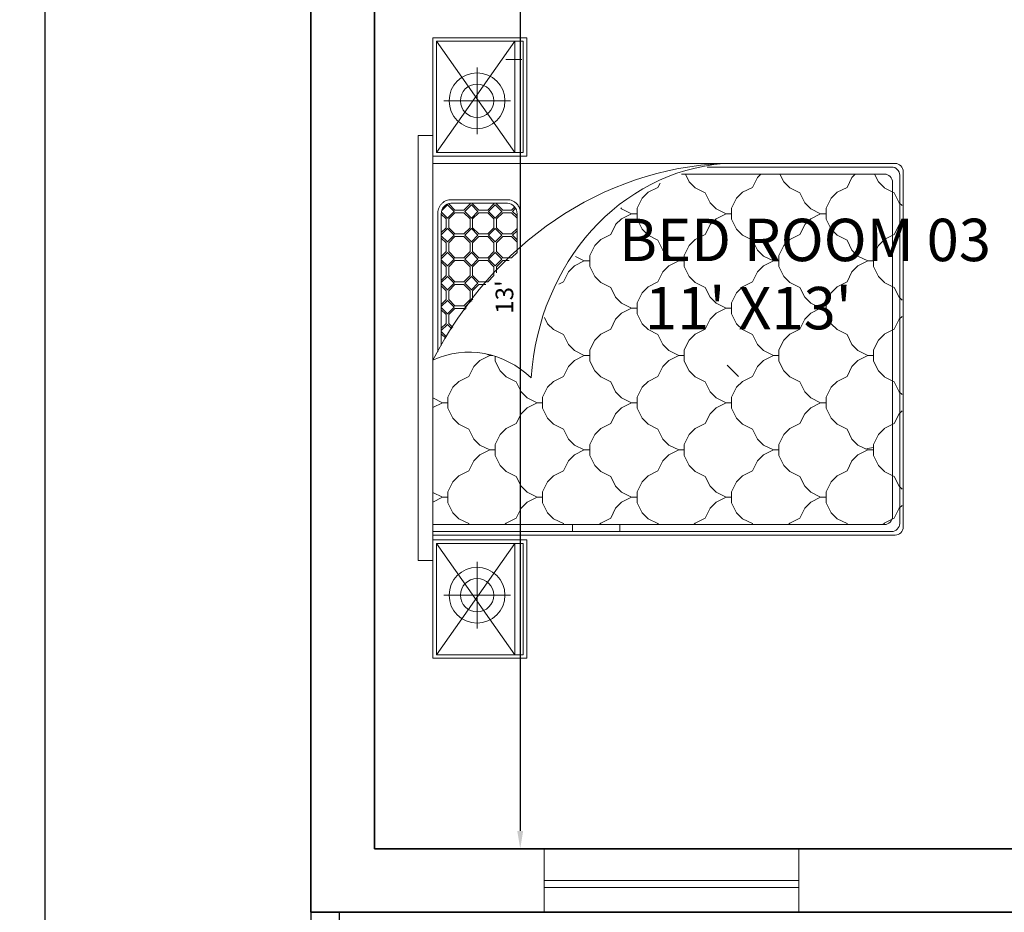
# Model space of a CAD drawing. Units: inches. Extents: x 2025 to 2528, y 1525 to 2336.
# Tile 2 of 18: x 2025 to 2164, y 1704 to 1831. Entities that reach past the tile are written whole.
import ezdxf

# ---------------------------------------------------------------- set-up
doc = ezdxf.new("R2010")
doc.units = ezdxf.units.IN
for name, color, linetype, lineweight in [('A-ANNO-DIMS', 2, 'Continuous', 18), ('A-AREA-IDEN', 7, 'Continuous', 25), ('A-FLOR', 7, 'Continuous', 25), ('A-FURN', 8, 'Continuous', 18), ('A-GLAZ', 4, 'Continuous', 18), ('A-WALL', 7, 'Continuous', 35)]:
    doc.layers.add(name, color=color, linetype=linetype, lineweight=lineweight)
doc.styles.get("Standard").update_dxf_attribs({"font": 'arial.ttf'})
doc.dimstyles.new('Copy of ISO-25', dxfattribs={"dimtxt": 2.5, "dimasz": 2.5, "dimexe": 1.25, "dimexo": 0.625, "dimtad": 1, "dimdec": 1, "dimlunit": 4, "dimtxsty": 'Standard', "dimcen": 2.5, "dimadec": 0, "dimazin": 0, "dimtfac": 1, "dimtdec": 1, "dimtmove": 0, "dimatfit": 3, "dimfxl": 1, "dimarcsym": 0})

# ---------------------------------------------------------------- blocks, each defined once
blk = doc.blocks.new('*D30')
at = {"layer": 'A-ANNO-DIMS', "color": 0, "lineweight": -2, "transparency": 16777216}
for p, q in [((2078.14, 1869.41), (2096.86, 1869.41)), ((2095.61, 1866.91), (2095.61, 1715.91)), ((2075.64, 1713.41), (2096.86, 1713.41))]:
    blk.add_line(p, q, dxfattribs=at)
at = {"layer": 'A-ANNO-DIMS', "color": 0, "transparency": 16777216}
for points in [[(2095.2, 1866.91), (2096.03, 1866.91), (2095.61, 1869.41)], [(2095.2, 1715.91), (2096.03, 1715.91), (2095.61, 1713.41)]]:
    blk.add_solid(points, dxfattribs=at)
at = {"layer": 'Defpoints', "color": 0, "transparency": 16777216}
for p in [(2077.51, 1869.41), (2075.01, 1713.41), (2095.61, 1713.41)]:
    blk.add_point(p, dxfattribs=at)
at = {"layer": 'A-ANNO-DIMS', "color": 0, "transparency": 16777216, "insert": (2093.71, 1791.41), "char_height": 2.5, "attachment_point": 5, "rotation": 90}
blk.add_mtext("13'", dxfattribs=at)
blk = doc.blocks.new('A$C029D5C69')
for p, q in [((0.4164, 2.0693), (0.4164, 2.0066)), ((2.2315, 2.0693), (0.4164, 2.0693)), ((2.2315, 2.0066), (2.2315, 2.0693)), ((0, 1.606), (0, 2.0066)), ((0, 2.0066), (0.505, 2.0066)), ((0.0151, 1.6211), (0.0151, 1.9915)), ((0.0151, 1.9915), (0.4899, 1.9915)), ((0.4164, 2.0066), (2.2315, 2.0066)), ((0.4899, 1.9915), (0.4899, 1.6211)), ((0.505, 2.0066), (0.505, 1.606)), ((0.5252, 0.0351), (0.5252, 2.0066)), ((0.5403, 0.0502), (0.5403, 2.0066)), ((0.5706, 0.0805), (0.5706, 2.0066)), ((0.6869, 1.966), (0.6666, 2.0066)), ((0.7072, 2.0066), (0.6869, 1.966)), ((1.0902, 1.966), (1.0699, 2.0066)), ((1.1106, 2.0066), (1.0902, 1.966)), ((1.8954, 1.9865), (1.3081, 1.9865)), ((2.1114, 2.0087), (2.1114, 0.0351)), ((2.6479, 2.0066), (2.1429, 2.0066)), ((2.1429, 2.0066), (2.1429, 1.606)), ((2.6328, 1.9915), (2.158, 1.9915)), ((2.158, 1.9915), (2.158, 1.6211)), ((2.6328, 1.6211), (2.6328, 1.9915)), ((2.6479, 1.606), (2.6479, 2.0066)), ((0.2689, 1.9609), (0.2689, 1.6764)), ((0.6634, 1.9425), (0.621, 1.9213)), ((0.6634, 1.9425), (0.621, 1.9213)), ((0.6869, 1.9425), (0.6634, 1.9425)), ((0.6869, 1.9425), (0.6869, 1.966)), ((0.6869, 1.9425), (0.6869, 1.966)), ((0.6869, 1.9425), (0.7104, 1.9425)), ((0.7528, 1.9213), (0.7104, 1.9425)), ((0.7528, 1.9213), (0.7104, 1.9425)), ((1.0668, 1.9425), (1.0244, 1.9213)), ((1.0668, 1.9425), (1.0244, 1.9213)), ((1.0902, 1.9425), (1.0668, 1.9425)), ((1.0902, 1.9425), (1.0902, 1.966)), ((1.0902, 1.9425), (1.0902, 1.966)), ((1.0902, 1.9425), (1.1137, 1.9425)), ((1.1561, 1.9213), (1.1137, 1.9425)), ((1.1561, 1.9213), (1.1137, 1.9425)), ((1.8954, 1.9713), (1.3339, 1.9713)), ((1.3849, 1.9713), (1.3656, 1.952)), ((1.3945, 1.9713), (1.3714, 1.9483)), ((1.4249, 1.945), (1.3986, 1.9713)), ((1.4249, 1.945), (1.4059, 1.926)), ((1.4288, 1.9507), (1.4081, 1.9713)), ((1.4288, 1.9394), (1.4116, 1.9222)), ((1.4476, 1.9507), (1.4288, 1.9507)), ((1.4288, 1.9393), (1.4476, 1.9393)), ((1.4476, 1.9507), (1.4664, 1.9507)), ((1.4664, 1.9393), (1.4476, 1.9393)), ((1.487, 1.9713), (1.4664, 1.9507)), ((1.493, 1.9128), (1.4664, 1.9394)), ((1.4966, 1.9713), (1.4703, 1.945)), ((1.4986, 1.9167), (1.4703, 1.945)), ((1.527, 1.945), (1.4986, 1.9167)), ((1.527, 1.945), (1.5007, 1.9713)), ((1.5309, 1.9394), (1.5043, 1.9128)), ((1.5309, 1.9507), (1.5102, 1.9713)), ((1.5497, 1.9507), (1.5309, 1.9507)), ((1.5309, 1.9393), (1.5497, 1.9393)), ((1.5497, 1.9507), (1.5685, 1.9507)), ((1.5685, 1.9393), (1.5497, 1.9393)), ((1.5891, 1.9713), (1.5685, 1.9507)), ((1.595, 1.9128), (1.5685, 1.9394)), ((1.5987, 1.9713), (1.5724, 1.945)), ((1.6007, 1.9167), (1.5724, 1.945)), ((1.6291, 1.945), (1.6007, 1.9167)), ((1.6291, 1.945), (1.6028, 1.9713)), ((1.633, 1.9394), (1.6064, 1.9128)), ((1.633, 1.9507), (1.6123, 1.9713)), ((1.6518, 1.9507), (1.633, 1.9507)), ((1.633, 1.9393), (1.6518, 1.9393)), ((1.6518, 1.9507), (1.6706, 1.9507)), ((1.6706, 1.9393), (1.6518, 1.9393)), ((1.6912, 1.9713), (1.6706, 1.9507)), ((1.6971, 1.9128), (1.6706, 1.9394)), ((1.7008, 1.9713), (1.6745, 1.945)), ((1.7028, 1.9167), (1.6745, 1.945)), ((1.7312, 1.945), (1.7028, 1.9167)), ((1.7312, 1.945), (1.7049, 1.9713)), ((1.7351, 1.9394), (1.7085, 1.9128)), ((1.7351, 1.9507), (1.7144, 1.9713)), ((1.7539, 1.9507), (1.7351, 1.9507)), ((1.7351, 1.9393), (1.7539, 1.9393)), ((1.7539, 1.9507), (1.7727, 1.9507)), ((1.7727, 1.9393), (1.7539, 1.9393)), ((1.7933, 1.9713), (1.7727, 1.9507)), ((1.7992, 1.9128), (1.7727, 1.9394)), ((1.8029, 1.9713), (1.7766, 1.945)), ((1.8049, 1.9167), (1.7766, 1.945)), ((1.8333, 1.945), (1.8049, 1.9167)), ((1.8333, 1.945), (1.807, 1.9713)), ((1.8372, 1.9394), (1.8106, 1.9128)), ((1.8372, 1.9507), (1.8165, 1.9713)), ((1.856, 1.9507), (1.8372, 1.9507)), ((1.8372, 1.9393), (1.856, 1.9393)), ((1.856, 1.9507), (1.8748, 1.9507)), ((1.8748, 1.9393), (1.856, 1.9393)), ((1.8954, 1.9713), (1.8748, 1.9507)), ((1.9013, 1.9128), (1.8748, 1.9394)), ((1.9043, 1.9707), (1.8787, 1.945)), ((1.907, 1.9167), (1.8787, 1.945)), ((1.9354, 1.945), (1.907, 1.9167)), ((1.9354, 1.945), (1.9114, 1.969)), ((1.9393, 1.9394), (1.9127, 1.9128)), ((1.9393, 1.9393), (1.9404, 1.9393)), ((2.379, 1.9609), (2.379, 1.6764)), ((0.5955, 1.8958), (0.5743, 1.8534)), ((0.621, 1.9213), (0.5955, 1.8958)), ((0.7783, 1.8958), (0.7528, 1.9213)), ((0.7995, 1.8534), (0.7783, 1.8958)), ((0.9989, 1.8958), (0.9777, 1.8534)), ((1.0243, 1.9213), (0.9988, 1.8958)), ((1.1816, 1.8958), (1.1561, 1.9213)), ((1.2028, 1.8534), (1.1816, 1.8958)), ((1.493, 1.8752), (1.493, 1.9128)), ((1.5043, 1.8752), (1.5043, 1.9128)), ((1.595, 1.8752), (1.595, 1.9128)), ((1.6064, 1.8752), (1.6064, 1.9128)), ((1.6971, 1.8752), (1.6971, 1.9128)), ((1.7085, 1.8752), (1.7085, 1.9128)), ((1.7992, 1.8752), (1.7992, 1.9128)), ((1.8106, 1.8752), (1.8106, 1.9128)), ((1.9013, 1.8752), (1.9013, 1.9128)), ((1.9127, 1.8752), (1.9127, 1.9128)), ((1.9414, 1.688), (1.9414, 1.931)), ((1.9565, 1.688), (1.9565, 1.931)), ((0.5743, 1.8534), (0.5706, 1.8515)), ((0.5743, 1.8534), (0.5706, 1.8515)), ((0.8419, 1.8322), (0.7995, 1.8534)), ((0.8419, 1.8322), (0.7995, 1.8534)), ((0.9777, 1.8534), (0.9353, 1.8322)), ((0.9777, 1.8534), (0.9353, 1.8322)), ((1.2452, 1.8322), (1.2028, 1.8534)), ((1.2452, 1.8322), (1.2028, 1.8534)), ((1.493, 1.8752), (1.4867, 1.869)), ((1.4986, 1.8713), (1.4922, 1.8648)), ((1.527, 1.8429), (1.4986, 1.8713)), ((1.5309, 1.8486), (1.5043, 1.8752)), ((1.5497, 1.8486), (1.5309, 1.8486)), ((1.5497, 1.8486), (1.5685, 1.8486)), ((1.595, 1.8752), (1.5685, 1.8486)), ((1.6007, 1.8713), (1.5724, 1.8429)), ((1.6291, 1.8429), (1.6007, 1.8713)), ((1.633, 1.8486), (1.6064, 1.8752)), ((1.6518, 1.8486), (1.633, 1.8486)), ((1.6518, 1.8486), (1.6706, 1.8486)), ((1.6971, 1.8752), (1.6706, 1.8486)), ((1.7028, 1.8713), (1.6745, 1.8429)), ((1.7312, 1.8429), (1.7028, 1.8713)), ((1.7351, 1.8486), (1.7085, 1.8752)), ((1.7539, 1.8486), (1.7351, 1.8486)), ((1.7539, 1.8486), (1.7727, 1.8486)), ((1.7992, 1.8752), (1.7727, 1.8486)), ((1.8049, 1.8713), (1.7766, 1.8429)), ((1.8333, 1.8429), (1.8049, 1.8713)), ((1.8372, 1.8486), (1.8106, 1.8752)), ((1.856, 1.8486), (1.8372, 1.8486)), ((1.856, 1.8486), (1.8748, 1.8486)), ((1.9013, 1.8752), (1.8748, 1.8486)), ((1.907, 1.8713), (1.8787, 1.8429)), ((1.9354, 1.8429), (1.907, 1.8713)), ((1.9393, 1.8486), (1.9127, 1.8752)), ((1.9414, 1.8486), (1.9393, 1.8486)), ((0.1267, 1.8186), (0.4111, 1.8186)), ((0.8674, 1.8067), (0.8419, 1.8322)), ((0.8886, 1.7643), (0.8674, 1.8067)), ((0.9098, 1.8067), (0.8886, 1.7643)), ((0.9352, 1.8322), (0.9097, 1.8067)), ((1.2707, 1.8067), (1.2452, 1.8322)), ((1.2919, 1.7643), (1.2707, 1.8067)), ((1.527, 1.8429), (1.5242, 1.8401)), ((1.5309, 1.8373), (1.5295, 1.8359)), ((1.5309, 1.8373), (1.5497, 1.8373)), ((1.5685, 1.8373), (1.5497, 1.8373)), ((1.595, 1.8107), (1.5685, 1.8373)), ((1.6007, 1.8146), (1.5724, 1.8429)), ((1.595, 1.7806), (1.595, 1.8107)), ((1.6291, 1.8429), (1.6007, 1.8146)), ((1.633, 1.8373), (1.6064, 1.8107)), ((1.6064, 1.7731), (1.6064, 1.8107)), ((1.633, 1.8373), (1.6518, 1.8373)), ((1.6706, 1.8373), (1.6518, 1.8373)), ((1.6971, 1.8107), (1.6706, 1.8373)), ((1.7028, 1.8146), (1.6745, 1.8429)), ((1.6971, 1.7731), (1.6971, 1.8107)), ((1.7312, 1.8429), (1.7028, 1.8146)), ((1.7351, 1.8373), (1.7085, 1.8107)), ((1.7085, 1.7731), (1.7085, 1.8107)), ((1.7351, 1.8373), (1.7539, 1.8373)), ((1.7727, 1.8373), (1.7539, 1.8373)), ((1.7992, 1.8107), (1.7727, 1.8373)), ((1.8049, 1.8146), (1.7766, 1.8429)), ((1.7992, 1.7731), (1.7992, 1.8107)), ((1.8333, 1.8429), (1.8049, 1.8146)), ((1.8372, 1.8373), (1.8106, 1.8107)), ((1.8106, 1.7731), (1.8106, 1.8107)), ((1.8372, 1.8373), (1.856, 1.8373)), ((1.8748, 1.8373), (1.856, 1.8373)), ((1.9013, 1.8107), (1.8748, 1.8373)), ((1.907, 1.8146), (1.8787, 1.8429)), ((1.9013, 1.7731), (1.9013, 1.8107)), ((1.9354, 1.8429), (1.907, 1.8146)), ((1.9393, 1.8373), (1.9127, 1.8107)), ((1.9127, 1.7731), (1.9127, 1.8107)), ((1.9393, 1.8373), (1.9414, 1.8373)), ((2.2367, 1.8186), (2.5212, 1.8186)), ((1.2981, 1.7768), (1.2919, 1.7643)), ((1.633, 1.7465), (1.6064, 1.7731)), ((1.6971, 1.7731), (1.6706, 1.7465)), ((1.7028, 1.7692), (1.6745, 1.7408)), ((1.7312, 1.7408), (1.7028, 1.7692)), ((1.7351, 1.7465), (1.7085, 1.7731)), ((1.7992, 1.7731), (1.7727, 1.7465)), ((1.8049, 1.7692), (1.7766, 1.7408)), ((1.8333, 1.7408), (1.8049, 1.7692)), ((1.8372, 1.7465), (1.8106, 1.7731)), ((1.9013, 1.7731), (1.8748, 1.7465)), ((1.907, 1.7692), (1.8787, 1.7408)), ((1.9354, 1.7408), (1.907, 1.7692)), ((1.9393, 1.7465), (1.9127, 1.7731)), ((0.8651, 1.7408), (0.8227, 1.7196)), ((0.8651, 1.7408), (0.8227, 1.7196)), ((0.912, 1.7408), (0.8651, 1.7408)), ((0.8886, 1.7408), (0.8886, 1.7643)), ((0.9544, 1.7196), (0.912, 1.7408)), ((0.9544, 1.7196), (0.912, 1.7408)), ((1.2684, 1.7408), (1.226, 1.7196)), ((1.2684, 1.7408), (1.226, 1.7196)), ((1.2885, 1.7408), (1.2684, 1.7408)), ((1.2919, 1.7519), (1.2919, 1.7643)), ((1.6518, 1.7465), (1.633, 1.7465)), ((1.6443, 1.7352), (1.6518, 1.7352)), ((1.6518, 1.7465), (1.6706, 1.7465)), ((1.6706, 1.7352), (1.6518, 1.7352)), ((1.6971, 1.7086), (1.6706, 1.7352)), ((1.7028, 1.7125), (1.6745, 1.7408)), ((1.7312, 1.7408), (1.7028, 1.7125)), ((1.7351, 1.7352), (1.7085, 1.7086)), ((1.7539, 1.7465), (1.7351, 1.7465)), ((1.7351, 1.7352), (1.7539, 1.7352)), ((1.7539, 1.7465), (1.7727, 1.7465)), ((1.7727, 1.7352), (1.7539, 1.7352)), ((1.7992, 1.7086), (1.7727, 1.7352)), ((1.8049, 1.7125), (1.7766, 1.7408)), ((1.8333, 1.7408), (1.8049, 1.7125)), ((1.8372, 1.7352), (1.8106, 1.7086)), ((1.856, 1.7465), (1.8372, 1.7465)), ((1.8372, 1.7352), (1.856, 1.7352)), ((1.856, 1.7465), (1.8748, 1.7465)), ((1.8748, 1.7352), (1.856, 1.7352)), ((1.9013, 1.7086), (1.8748, 1.7352)), ((1.907, 1.7125), (1.8787, 1.7408)), ((1.9354, 1.7408), (1.907, 1.7125)), ((1.9393, 1.7352), (1.9127, 1.7086)), ((1.9414, 1.7465), (1.9393, 1.7465)), ((1.9393, 1.7352), (1.9414, 1.7352)), ((0.5766, 1.6941), (0.5706, 1.7002)), ((0.5978, 1.6517), (0.5766, 1.6941)), ((0.7972, 1.6941), (0.776, 1.6517)), ((0.8227, 1.7196), (0.7972, 1.6941)), ((0.98, 1.6941), (0.9545, 1.7196)), ((1.0011, 1.6517), (0.9799, 1.6941)), ((1.2005, 1.6941), (1.1793, 1.6517)), ((1.226, 1.7196), (1.2005, 1.6941)), ((1.6971, 1.682), (1.6971, 1.7086)), ((1.7085, 1.671), (1.7085, 1.7086)), ((1.7992, 1.671), (1.7992, 1.7086)), ((1.8106, 1.671), (1.8106, 1.7086)), ((1.9013, 1.671), (1.9013, 1.7086)), ((1.9127, 1.671), (1.9127, 1.7086)), ((2.5551, 1.6275), (2.5551, 1.696)), ((0.6402, 1.6305), (0.5978, 1.6517)), ((0.6402, 1.6305), (0.5978, 1.6517)), ((0.776, 1.6517), (0.7336, 1.6305)), ((0.776, 1.6517), (0.7336, 1.6305)), ((1.0435, 1.6305), (1.0011, 1.6517)), ((1.0435, 1.6305), (1.0011, 1.6517)), ((1.1793, 1.6517), (1.1369, 1.6305)), ((1.1793, 1.6517), (1.1369, 1.6305)), ((1.7318, 1.6477), (1.7085, 1.671)), ((1.8961, 1.6477), (1.7289, 1.6477)), ((1.7992, 1.671), (1.7759, 1.6477)), ((1.8049, 1.6671), (1.7855, 1.6477)), ((1.8244, 1.6477), (1.8049, 1.6671)), ((1.8339, 1.6477), (1.8106, 1.671)), ((1.9013, 1.671), (1.878, 1.6477)), ((1.907, 1.6671), (1.8876, 1.6477)), ((1.9202, 1.6539), (1.907, 1.6671)), ((1.926, 1.6577), (1.9127, 1.671)), ((0.505, 1.606), (0, 1.606)), ((0.4899, 1.6211), (0.0151, 1.6211)), ((0.6657, 1.605), (0.6402, 1.6305)), ((0.6869, 1.5626), (0.6657, 1.605)), ((0.7081, 1.605), (0.6869, 1.5626)), ((0.7336, 1.6305), (0.7081, 1.605)), ((1.0691, 1.605), (1.0436, 1.6305)), ((1.0902, 1.5626), (1.069, 1.605)), ((1.1114, 1.605), (1.0902, 1.5626)), ((1.1369, 1.6305), (1.1114, 1.605)), ((1.8961, 1.6325), (1.7422, 1.6325)), ((2.1429, 1.606), (2.6479, 1.606)), ((2.158, 1.6211), (2.6328, 1.6211)), ((0.6869, 1.5392), (0.6869, 1.5626)), ((0.6869, 1.5392), (0.6869, 1.5626)), ((1.0902, 1.5392), (1.0902, 1.5626)), ((1.0902, 1.5392), (1.0902, 1.5626)), ((0.621, 1.5179), (0.5955, 1.4924)), ((0.6634, 1.5391), (0.621, 1.5179)), ((0.6634, 1.5391), (0.621, 1.5179)), ((0.6869, 1.5392), (0.6634, 1.5392)), ((0.6869, 1.5392), (0.7104, 1.5392)), ((0.7528, 1.5179), (0.7104, 1.5391)), ((0.7528, 1.5179), (0.7104, 1.5391)), ((0.7783, 1.4924), (0.7528, 1.5179)), ((1.0243, 1.5179), (0.9988, 1.4924)), ((1.0668, 1.5391), (1.0244, 1.5179)), ((1.0668, 1.5391), (1.0244, 1.5179)), ((1.0902, 1.5392), (1.0668, 1.5392)), ((1.0902, 1.5392), (1.1137, 1.5392)), ((1.1561, 1.5179), (1.1137, 1.5391)), ((1.1561, 1.5179), (1.1137, 1.5391)), ((1.1816, 1.4924), (1.1561, 1.5179)), ((1.4277, 1.5179), (1.4022, 1.4924)), ((1.4534, 1.5308), (1.4277, 1.5179)), ((1.4534, 1.5308), (1.4277, 1.5179)), ((0.5955, 1.4925), (0.5743, 1.4501)), ((0.7995, 1.4501), (0.7783, 1.4925)), ((0.9989, 1.4925), (0.9777, 1.4501)), ((1.2028, 1.4501), (1.1816, 1.4925)), ((1.4022, 1.4925), (1.381, 1.4501)), ((0.5743, 1.45), (0.5706, 1.4481)), ((0.5743, 1.45), (0.5706, 1.4481)), ((0.8419, 1.4288), (0.7995, 1.45)), ((0.8419, 1.4288), (0.7995, 1.45)), ((0.8674, 1.4033), (0.8419, 1.4288)), ((0.9352, 1.4288), (0.9097, 1.4033)), ((0.9777, 1.45), (0.9353, 1.4288)), ((0.9777, 1.45), (0.9353, 1.4288)), ((1.2452, 1.4288), (1.2028, 1.45)), ((1.2452, 1.4288), (1.2028, 1.45)), ((1.2707, 1.4033), (1.2452, 1.4288)), ((1.3386, 1.4288), (1.3131, 1.4033)), ((1.381, 1.45), (1.3386, 1.4288)), ((1.381, 1.45), (1.3386, 1.4288)), ((1.6062, 1.4501), (1.5966, 1.4692)), ((1.6486, 1.4288), (1.6062, 1.45)), ((1.6486, 1.4288), (1.6062, 1.45)), ((1.6741, 1.4033), (1.6486, 1.4288)), ((0.5403, 1.4117), (0.5706, 1.4117)), ((0.8886, 1.361), (0.8674, 1.4034)), ((0.9098, 1.4034), (0.8886, 1.361)), ((1.2919, 1.361), (1.2707, 1.4034)), ((1.3131, 1.4034), (1.2919, 1.361)), ((1.6953, 1.361), (1.6741, 1.4034)), ((1.714, 1.3984), (1.6953, 1.361)), ((0.8886, 1.3375), (0.8886, 1.3609)), ((1.2919, 1.3375), (1.2919, 1.3609)), ((1.6953, 1.3375), (1.6953, 1.3609)), ((0.8227, 1.3163), (0.7972, 1.2908)), ((0.8651, 1.3374), (0.8227, 1.3162)), ((0.8651, 1.3374), (0.8227, 1.3162)), ((0.912, 1.3375), (0.8651, 1.3375)), ((0.9544, 1.3162), (0.912, 1.3374)), ((0.9544, 1.3162), (0.912, 1.3374)), ((0.98, 1.2908), (0.9545, 1.3163)), ((1.226, 1.3163), (1.2005, 1.2908)), ((1.2684, 1.3374), (1.226, 1.3162)), ((1.2684, 1.3374), (1.226, 1.3162)), ((1.3154, 1.3375), (1.2684, 1.3375)), ((1.3578, 1.3162), (1.3154, 1.3374)), ((1.3578, 1.3162), (1.3154, 1.3374)), ((1.3833, 1.2908), (1.3578, 1.3163)), ((1.6294, 1.3163), (1.6039, 1.2908)), ((1.6718, 1.3374), (1.6294, 1.3162)), ((1.6718, 1.3374), (1.6294, 1.3162)), ((1.7187, 1.3375), (1.6718, 1.3375)), ((1.7611, 1.3162), (1.7187, 1.3374)), ((1.7611, 1.3162), (1.7187, 1.3374)), ((1.7867, 1.2908), (1.7611, 1.3163)), ((0.5766, 1.2908), (0.5706, 1.2968)), ((0.5978, 1.2484), (0.5766, 1.2908)), ((0.7972, 1.2908), (0.776, 1.2484)), ((1.0011, 1.2484), (0.9799, 1.2908)), ((1.2005, 1.2908), (1.1793, 1.2484)), ((1.4045, 1.2484), (1.3833, 1.2908)), ((1.6039, 1.2908), (1.5827, 1.2484)), ((1.8078, 1.2484), (1.7866, 1.2908)), ((0.6402, 1.2271), (0.5978, 1.2483)), ((0.6402, 1.2271), (0.5978, 1.2483)), ((0.6657, 1.2017), (0.6402, 1.2272)), ((0.7336, 1.2272), (0.7081, 1.2017)), ((0.776, 1.2483), (0.7336, 1.2271)), ((0.776, 1.2483), (0.7336, 1.2271)), ((1.0435, 1.2271), (1.0011, 1.2483)), ((1.0435, 1.2271), (1.0011, 1.2483)), ((1.0691, 1.2017), (1.0436, 1.2272)), ((1.1369, 1.2272), (1.1114, 1.2017)), ((1.1793, 1.2483), (1.1369, 1.2271)), ((1.1793, 1.2483), (1.1369, 1.2271)), ((1.4469, 1.2271), (1.4045, 1.2483)), ((1.4469, 1.2271), (1.4045, 1.2483)), ((1.4724, 1.2017), (1.4469, 1.2272)), ((1.5403, 1.2272), (1.5148, 1.2017)), ((1.5827, 1.2483), (1.5403, 1.2271)), ((1.5827, 1.2483), (1.5403, 1.2271)), ((1.8502, 1.2271), (1.8078, 1.2483)), ((1.8502, 1.2271), (1.8078, 1.2483)), ((1.8758, 1.2017), (1.8503, 1.2272)), ((0.5403, 1.21), (0.5706, 1.21)), ((0.6869, 1.1593), (0.6657, 1.2017)), ((0.7081, 1.2017), (0.6869, 1.1593)), ((1.0902, 1.1593), (1.069, 1.2017)), ((1.1114, 1.2017), (1.0902, 1.1593)), ((1.4936, 1.1593), (1.4724, 1.2017)), ((1.5148, 1.2017), (1.4936, 1.1593)), ((1.8969, 1.1593), (1.8757, 1.2017)), ((1.9181, 1.2017), (1.8969, 1.1593)), ((1.9215, 1.2051), (1.9181, 1.2017)), ((0.6634, 1.1358), (0.621, 1.1146)), ((0.6634, 1.1358), (0.621, 1.1146)), ((0.6869, 1.1358), (0.6634, 1.1358)), ((0.6869, 1.1358), (0.6869, 1.1593)), ((0.6869, 1.1358), (0.6869, 1.1593)), ((0.6869, 1.1358), (0.7104, 1.1358)), ((0.7528, 1.1146), (0.7104, 1.1358)), ((0.7528, 1.1146), (0.7104, 1.1358)), ((1.0668, 1.1358), (1.0244, 1.1146)), ((1.0668, 1.1358), (1.0244, 1.1146)), ((1.0902, 1.1358), (1.0668, 1.1358)), ((1.0902, 1.1358), (1.0902, 1.1593)), ((1.0902, 1.1358), (1.0902, 1.1593)), ((1.0902, 1.1358), (1.1137, 1.1358)), ((1.1561, 1.1146), (1.1137, 1.1358)), ((1.1561, 1.1146), (1.1137, 1.1358)), ((1.4701, 1.1358), (1.4277, 1.1146)), ((1.4701, 1.1358), (1.4277, 1.1146)), ((1.4936, 1.1358), (1.4701, 1.1358)), ((1.4936, 1.1358), (1.4936, 1.1593)), ((1.4936, 1.1358), (1.4936, 1.1593)), ((1.4936, 1.1358), (1.5171, 1.1358)), ((1.5595, 1.1146), (1.5171, 1.1358)), ((1.5595, 1.1146), (1.5171, 1.1358)), ((1.8735, 1.1358), (1.8311, 1.1146)), ((1.8735, 1.1358), (1.8311, 1.1146)), ((1.8969, 1.1358), (1.8735, 1.1358)), ((1.8969, 1.1358), (1.8969, 1.1593)), ((1.8969, 1.1358), (1.8969, 1.1593)), ((1.8969, 1.1358), (1.9204, 1.1358)), ((1.9628, 1.1146), (1.9204, 1.1358)), ((1.9628, 1.1146), (1.9204, 1.1358)), ((0.621, 1.1146), (0.5955, 1.0891)), ((0.7783, 1.0891), (0.7528, 1.1146)), ((1.0243, 1.1146), (0.9988, 1.0891)), ((1.1816, 1.0891), (1.1561, 1.1146)), ((1.4277, 1.1146), (1.4022, 1.0891)), ((1.585, 1.0891), (1.5595, 1.1146)), ((1.831, 1.1146), (1.8055, 1.0891)), ((1.9883, 1.0891), (1.9628, 1.1146)), ((0.5955, 1.0891), (0.5743, 1.0467)), ((0.7995, 1.0467), (0.7783, 1.0891)), ((0.9989, 1.0891), (0.9777, 1.0467)), ((1.2028, 1.0467), (1.1816, 1.0891)), ((1.4022, 1.0891), (1.381, 1.0467)), ((1.6062, 1.0467), (1.585, 1.0891)), ((1.8056, 1.0891), (1.7844, 1.0467)), ((2.0095, 1.0467), (1.9883, 1.0891)), ((0.5743, 1.0467), (0.5706, 1.0448)), ((0.5743, 1.0467), (0.5706, 1.0448)), ((0.8419, 1.0255), (0.7995, 1.0467)), ((0.8419, 1.0255), (0.7995, 1.0467)), ((0.8674, 1), (0.8419, 1.0255)), ((0.9352, 1.0255), (0.9097, 1)), ((0.9777, 1.0467), (0.9353, 1.0255)), ((0.9777, 1.0467), (0.9353, 1.0255)), ((1.2452, 1.0255), (1.2028, 1.0467)), ((1.2452, 1.0255), (1.2028, 1.0467)), ((1.2707, 1), (1.2452, 1.0255)), ((1.3386, 1.0255), (1.3131, 1)), ((1.381, 1.0467), (1.3386, 1.0255)), ((1.381, 1.0467), (1.3386, 1.0255)), ((1.6486, 1.0255), (1.6062, 1.0467)), ((1.6486, 1.0255), (1.6062, 1.0467)), ((1.6741, 1), (1.6486, 1.0255)), ((1.7419, 1.0255), (1.7164, 1)), ((1.7844, 1.0467), (1.742, 1.0255)), ((1.7844, 1.0467), (1.742, 1.0255)), ((2.0276, 1.0376), (2.0095, 1.0467)), ((2.0276, 1.0376), (2.0095, 1.0467)), ((0.8886, 0.9576), (0.8674, 1)), ((0.9098, 1), (0.8886, 0.9576)), ((1.2919, 0.9576), (1.2707, 1)), ((1.3131, 1), (1.2919, 0.9576)), ((1.6953, 0.9576), (1.6741, 1)), ((1.7165, 1), (1.6953, 0.9576)), ((0.8651, 0.9341), (0.8227, 0.9129)), ((0.8651, 0.9341), (0.8227, 0.9129)), ((0.912, 0.9341), (0.8651, 0.9341)), ((0.8886, 0.9341), (0.8886, 0.9576)), ((0.9544, 0.9129), (0.912, 0.9341)), ((0.9544, 0.9129), (0.912, 0.9341)), ((1.2684, 0.9341), (1.226, 0.9129)), ((1.2684, 0.9341), (1.226, 0.9129)), ((1.3154, 0.9341), (1.2684, 0.9341)), ((1.2919, 0.9341), (1.2919, 0.9576)), ((1.3578, 0.9129), (1.3154, 0.9341)), ((1.3578, 0.9129), (1.3154, 0.9341)), ((1.6718, 0.9341), (1.6294, 0.9129)), ((1.6718, 0.9341), (1.6294, 0.9129)), ((1.7187, 0.9341), (1.6718, 0.9341)), ((1.6953, 0.9341), (1.6953, 0.9576)), ((1.7611, 0.9129), (1.7187, 0.9341)), ((1.7611, 0.9129), (1.7187, 0.9341)), ((2.066, 0.9295), (2.0327, 0.9129)), ((2.066, 0.9295), (2.0327, 0.9129)), ((2.066, 0.9457), (2.066, 0.0805)), ((0.5766, 0.8874), (0.5706, 0.8935)), ((0.5978, 0.845), (0.5766, 0.8874)), ((0.7972, 0.8874), (0.776, 0.845)), ((0.8227, 0.9129), (0.7972, 0.8874)), ((0.98, 0.8874), (0.9545, 0.9129)), ((1.0011, 0.845), (0.9799, 0.8874)), ((1.2005, 0.8874), (1.1793, 0.845)), ((1.226, 0.9129), (1.2005, 0.8874)), ((1.3833, 0.8874), (1.3578, 0.9129)), ((1.4045, 0.845), (1.3833, 0.8874)), ((1.6039, 0.8874), (1.5827, 0.845)), ((1.6294, 0.9129), (1.6039, 0.8874)), ((1.7867, 0.8874), (1.7611, 0.9129)), ((1.8078, 0.845), (1.7866, 0.8874)), ((2.0072, 0.8874), (1.986, 0.845)), ((2.0327, 0.9129), (2.0072, 0.8874)), ((0.6402, 0.8238), (0.5978, 0.845)), ((0.6402, 0.8238), (0.5978, 0.845)), ((0.776, 0.845), (0.7336, 0.8238)), ((0.776, 0.845), (0.7336, 0.8238)), ((1.0435, 0.8238), (1.0011, 0.845)), ((1.0435, 0.8238), (1.0011, 0.845)), ((1.1793, 0.845), (1.1369, 0.8238)), ((1.1793, 0.845), (1.1369, 0.8238)), ((1.4469, 0.8238), (1.4045, 0.845)), ((1.4469, 0.8238), (1.4045, 0.845)), ((1.5827, 0.845), (1.5403, 0.8238)), ((1.5827, 0.845), (1.5403, 0.8238)), ((1.8502, 0.8238), (1.8078, 0.845)), ((1.8502, 0.8238), (1.8078, 0.845)), ((1.986, 0.845), (1.9436, 0.8238)), ((1.986, 0.845), (1.9436, 0.8238)), ((0.6657, 0.7983), (0.6402, 0.8238)), ((0.6869, 0.7559), (0.6657, 0.7983)), ((0.7081, 0.7983), (0.6869, 0.7559)), ((0.7336, 0.8238), (0.7081, 0.7983)), ((1.0691, 0.7983), (1.0436, 0.8238)), ((1.0902, 0.7559), (1.069, 0.7983)), ((1.1114, 0.7983), (1.0902, 0.7559)), ((1.1369, 0.8238), (1.1114, 0.7983)), ((1.4724, 0.7983), (1.4469, 0.8238)), ((1.4936, 0.7559), (1.4724, 0.7983)), ((1.5148, 0.7983), (1.4936, 0.7559)), ((1.5403, 0.8238), (1.5148, 0.7983)), ((1.8758, 0.7983), (1.8503, 0.8238)), ((1.8969, 0.7559), (1.8757, 0.7983)), ((1.9181, 0.7983), (1.8969, 0.7559)), ((1.9436, 0.8238), (1.9181, 0.7983)), ((2.0962, 0.8369), (2.0962, 0.0502)), ((0.6634, 0.7324), (0.621, 0.7112)), ((0.6634, 0.7324), (0.621, 0.7112)), ((0.6869, 0.7325), (0.6634, 0.7325)), ((0.6869, 0.7325), (0.6869, 0.7559)), ((0.6869, 0.7325), (0.6869, 0.7559)), ((0.6869, 0.7325), (0.7104, 0.7325)), ((0.7528, 0.7112), (0.7104, 0.7324)), ((0.7528, 0.7112), (0.7104, 0.7324)), ((1.0668, 0.7324), (1.0244, 0.7112)), ((1.0668, 0.7324), (1.0244, 0.7112)), ((1.0902, 0.7325), (1.0668, 0.7325)), ((1.0902, 0.7325), (1.0902, 0.7559)), ((1.0902, 0.7325), (1.0902, 0.7559)), ((1.0902, 0.7325), (1.1137, 0.7325)), ((1.1561, 0.7112), (1.1137, 0.7324)), ((1.1561, 0.7112), (1.1137, 0.7324)), ((1.2024, 0.7028), (1.2503, 0.7507)), ((1.4701, 0.7324), (1.4277, 0.7112)), ((1.4701, 0.7324), (1.4277, 0.7112)), ((1.4936, 0.7325), (1.4701, 0.7325)), ((1.4936, 0.7325), (1.4936, 0.7559)), ((1.4936, 0.7325), (1.4936, 0.7559)), ((1.4936, 0.7325), (1.5171, 0.7325)), ((1.5595, 0.7112), (1.5171, 0.7324)), ((1.5595, 0.7112), (1.5171, 0.7324)), ((1.8735, 0.7324), (1.8311, 0.7112)), ((1.8735, 0.7324), (1.8311, 0.7112)), ((1.8969, 0.7325), (1.8735, 0.7325)), ((1.8969, 0.7325), (1.8969, 0.7559)), ((1.8969, 0.7325), (1.8969, 0.7559)), ((1.8969, 0.7325), (1.9204, 0.7325)), ((1.9628, 0.7112), (1.9204, 0.7324)), ((1.9628, 0.7112), (1.9204, 0.7324)), ((0.5955, 0.6858), (0.5743, 0.6434)), ((0.621, 0.7113), (0.5955, 0.6858)), ((0.7783, 0.6858), (0.7528, 0.7113)), ((0.7995, 0.6434), (0.7783, 0.6858)), ((0.9989, 0.6858), (0.9777, 0.6434)), ((1.0243, 0.7113), (0.9988, 0.6858)), ((1.1816, 0.6858), (1.1561, 0.7113)), ((1.2028, 0.6434), (1.1816, 0.6858)), ((1.4022, 0.6858), (1.381, 0.6434)), ((1.4277, 0.7113), (1.4022, 0.6858)), ((1.585, 0.6858), (1.5595, 0.7113)), ((1.6062, 0.6434), (1.585, 0.6858)), ((1.8056, 0.6858), (1.7844, 0.6434)), ((1.831, 0.7113), (1.8055, 0.6858)), ((1.9883, 0.6858), (1.9628, 0.7113)), ((2.0095, 0.6434), (1.9883, 0.6858)), ((0.5743, 0.6433), (0.5706, 0.6414)), ((0.5743, 0.6433), (0.5706, 0.6414)), ((0.8419, 0.6221), (0.7995, 0.6433)), ((0.8419, 0.6221), (0.7995, 0.6433)), ((0.9777, 0.6433), (0.9353, 0.6221)), ((0.9777, 0.6433), (0.9353, 0.6221)), ((1.2452, 0.6221), (1.2028, 0.6433)), ((1.2452, 0.6221), (1.2028, 0.6433)), ((1.381, 0.6433), (1.3386, 0.6221)), ((1.381, 0.6433), (1.3386, 0.6221)), ((1.6486, 0.6221), (1.6062, 0.6433)), ((1.6486, 0.6221), (1.6062, 0.6433)), ((1.7844, 0.6433), (1.742, 0.6221)), ((1.7844, 0.6433), (1.742, 0.6221)), ((2.0519, 0.6221), (2.0095, 0.6433)), ((2.0519, 0.6221), (2.0095, 0.6433)), ((0.8674, 0.5967), (0.8419, 0.6222)), ((0.8886, 0.5543), (0.8674, 0.5967)), ((0.9098, 0.5967), (0.8886, 0.5543)), ((0.9352, 0.6222), (0.9097, 0.5967)), ((1.2707, 0.5967), (1.2452, 0.6222)), ((1.2919, 0.5543), (1.2707, 0.5967)), ((1.3131, 0.5967), (1.2919, 0.5543)), ((1.3386, 0.6222), (1.3131, 0.5967)), ((1.6741, 0.5967), (1.6486, 0.6222)), ((1.6953, 0.5543), (1.6741, 0.5967)), ((1.7165, 0.5967), (1.6953, 0.5543)), ((1.7419, 0.6222), (1.7164, 0.5967)), ((2.066, 0.6081), (2.0519, 0.6222)), ((0.8886, 0.5308), (0.8886, 0.5543)), ((1.2919, 0.5308), (1.2919, 0.5543)), ((1.6953, 0.5308), (1.6953, 0.5543)), ((0.8227, 0.5096), (0.7972, 0.4841)), ((0.8651, 0.5308), (0.8227, 0.5096)), ((0.8651, 0.5308), (0.8227, 0.5096)), ((0.912, 0.5308), (0.8651, 0.5308)), ((0.9544, 0.5096), (0.912, 0.5308)), ((0.9544, 0.5096), (0.912, 0.5308)), ((0.98, 0.4841), (0.9545, 0.5096)), ((1.226, 0.5096), (1.2005, 0.4841)), ((1.2684, 0.5308), (1.226, 0.5096)), ((1.2684, 0.5308), (1.226, 0.5096)), ((1.3154, 0.5308), (1.2684, 0.5308)), ((1.3578, 0.5096), (1.3154, 0.5308)), ((1.3578, 0.5096), (1.3154, 0.5308)), ((1.3833, 0.4841), (1.3578, 0.5096)), ((1.6294, 0.5096), (1.6039, 0.4841)), ((1.6718, 0.5308), (1.6294, 0.5096)), ((1.6718, 0.5308), (1.6294, 0.5096)), ((1.7187, 0.5308), (1.6718, 0.5308)), ((1.7611, 0.5096), (1.7187, 0.5308)), ((1.7611, 0.5096), (1.7187, 0.5308)), ((1.7867, 0.4841), (1.7611, 0.5096)), ((2.0327, 0.5096), (2.0072, 0.4841)), ((2.066, 0.5262), (2.0327, 0.5096)), ((2.066, 0.5262), (2.0327, 0.5096)), ((0.5766, 0.4841), (0.5706, 0.4901)), ((0.5978, 0.4417), (0.5766, 0.4841)), ((0.7972, 0.4841), (0.776, 0.4417)), ((1.0011, 0.4417), (0.9799, 0.4841)), ((1.2005, 0.4841), (1.1793, 0.4417)), ((1.4045, 0.4417), (1.3833, 0.4841)), ((1.6039, 0.4841), (1.5827, 0.4417)), ((1.8078, 0.4417), (1.7866, 0.4841)), ((2.0072, 0.4841), (1.986, 0.4417)), ((0.6402, 0.4205), (0.5978, 0.4417)), ((0.6402, 0.4205), (0.5978, 0.4417)), ((0.6657, 0.395), (0.6402, 0.4205)), ((0.7336, 0.4205), (0.7081, 0.395)), ((0.776, 0.4417), (0.7336, 0.4205)), ((0.776, 0.4417), (0.7336, 0.4205)), ((1.0435, 0.4205), (1.0011, 0.4417)), ((1.0435, 0.4205), (1.0011, 0.4417)), ((1.0691, 0.395), (1.0436, 0.4205)), ((1.1369, 0.4205), (1.1114, 0.395)), ((1.1793, 0.4417), (1.1369, 0.4205)), ((1.1793, 0.4417), (1.1369, 0.4205)), ((1.4469, 0.4205), (1.4045, 0.4417)), ((1.4469, 0.4205), (1.4045, 0.4417)), ((1.4724, 0.395), (1.4469, 0.4205)), ((1.5403, 0.4205), (1.5148, 0.395)), ((1.5827, 0.4417), (1.5403, 0.4205)), ((1.5827, 0.4417), (1.5403, 0.4205)), ((1.8502, 0.4205), (1.8078, 0.4417)), ((1.8502, 0.4205), (1.8078, 0.4417)), ((1.8758, 0.395), (1.8503, 0.4205)), ((1.9436, 0.4205), (1.9181, 0.395)), ((1.986, 0.4417), (1.9436, 0.4205)), ((1.986, 0.4417), (1.9436, 0.4205)), ((0.6869, 0.3526), (0.6657, 0.395)), ((0.7081, 0.395), (0.6869, 0.3526)), ((1.0902, 0.3526), (1.069, 0.395)), ((1.1114, 0.395), (1.0902, 0.3526)), ((1.4936, 0.3526), (1.4724, 0.395)), ((1.5148, 0.395), (1.4936, 0.3526)), ((1.8969, 0.3526), (1.8757, 0.395)), ((1.9181, 0.395), (1.8969, 0.3526)), ((0.6869, 0.3291), (0.6869, 0.3526)), ((0.6869, 0.3291), (0.6869, 0.3526)), ((1.0902, 0.3291), (1.0902, 0.3526)), ((1.0902, 0.3291), (1.0902, 0.3526)), ((1.4936, 0.3291), (1.4936, 0.3526)), ((1.4936, 0.3291), (1.4936, 0.3526)), ((1.8969, 0.3291), (1.8969, 0.3526)), ((1.8969, 0.3291), (1.8969, 0.3526)), ((0.621, 0.3079), (0.5955, 0.2824)), ((0.6634, 0.3291), (0.621, 0.3079)), ((0.6634, 0.3291), (0.621, 0.3079)), ((0.6869, 0.3291), (0.6634, 0.3291)), ((0.6869, 0.3291), (0.7104, 0.3291)), ((0.7528, 0.3079), (0.7104, 0.3291)), ((0.7528, 0.3079), (0.7104, 0.3291)), ((0.7783, 0.2824), (0.7528, 0.3079)), ((1.0243, 0.3079), (0.9988, 0.2824)), ((1.0668, 0.3291), (1.0244, 0.3079)), ((1.0668, 0.3291), (1.0244, 0.3079)), ((1.0902, 0.3291), (1.0668, 0.3291)), ((1.0902, 0.3291), (1.1137, 0.3291)), ((1.1561, 0.3079), (1.1137, 0.3291)), ((1.1561, 0.3079), (1.1137, 0.3291)), ((1.1816, 0.2824), (1.1561, 0.3079)), ((1.4277, 0.3079), (1.4022, 0.2824)), ((1.4701, 0.3291), (1.4277, 0.3079)), ((1.4701, 0.3291), (1.4277, 0.3079)), ((1.4936, 0.3291), (1.4701, 0.3291)), ((1.4936, 0.3291), (1.5171, 0.3291)), ((1.5595, 0.3079), (1.5171, 0.3291)), ((1.5595, 0.3079), (1.5171, 0.3291)), ((1.585, 0.2824), (1.5595, 0.3079)), ((1.831, 0.3079), (1.8055, 0.2824)), ((1.8735, 0.3291), (1.8311, 0.3079)), ((1.8735, 0.3291), (1.8311, 0.3079)), ((1.8969, 0.3291), (1.8735, 0.3291)), ((1.8969, 0.3291), (1.9204, 0.3291)), ((1.9628, 0.3079), (1.9204, 0.3291)), ((1.9628, 0.3079), (1.9204, 0.3291)), ((1.9883, 0.2824), (1.9628, 0.3079)), ((0.5955, 0.2824), (0.5743, 0.24)), ((0.7995, 0.24), (0.7783, 0.2824)), ((0.9989, 0.2824), (0.9777, 0.24)), ((1.2028, 0.24), (1.1816, 0.2824)), ((1.4022, 0.2824), (1.381, 0.24)), ((1.6062, 0.24), (1.585, 0.2824)), ((1.8056, 0.2824), (1.7844, 0.24)), ((2.0095, 0.24), (1.9883, 0.2824)), ((0.5743, 0.24), (0.5706, 0.2381)), ((0.5743, 0.24), (0.5706, 0.2381)), ((0.8419, 0.2188), (0.7995, 0.24)), ((0.8419, 0.2188), (0.7995, 0.24)), ((0.8674, 0.1933), (0.8419, 0.2188)), ((0.9352, 0.2188), (0.9097, 0.1933)), ((0.9777, 0.24), (0.9353, 0.2188)), ((0.9777, 0.24), (0.9353, 0.2188)), ((1.2452, 0.2188), (1.2028, 0.24)), ((1.2452, 0.2188), (1.2028, 0.24)), ((1.2707, 0.1933), (1.2452, 0.2188)), ((1.3386, 0.2188), (1.3131, 0.1933)), ((1.381, 0.24), (1.3386, 0.2188)), ((1.381, 0.24), (1.3386, 0.2188)), ((1.6486, 0.2188), (1.6062, 0.24)), ((1.6486, 0.2188), (1.6062, 0.24)), ((1.6741, 0.1933), (1.6486, 0.2188)), ((1.7419, 0.2188), (1.7164, 0.1933)), ((1.7844, 0.24), (1.742, 0.2188)), ((1.7844, 0.24), (1.742, 0.2188)), ((2.0519, 0.2188), (2.0095, 0.24)), ((2.0519, 0.2188), (2.0095, 0.24)), ((2.066, 0.2047), (2.0519, 0.2188)), ((0.8886, 0.1509), (0.8674, 0.1933)), ((0.9098, 0.1933), (0.8886, 0.1509)), ((1.2919, 0.1509), (1.2707, 0.1933)), ((1.3131, 0.1933), (1.2919, 0.1509)), ((1.6953, 0.1509), (1.6741, 0.1933)), ((1.7165, 0.1933), (1.6953, 0.1509)), ((0.8651, 0.1274), (0.8227, 0.1062)), ((0.8651, 0.1274), (0.8227, 0.1062)), ((0.912, 0.1275), (0.8651, 0.1275)), ((0.8886, 0.1275), (0.8886, 0.1509)), ((0.9544, 0.1062), (0.912, 0.1274)), ((0.9544, 0.1062), (0.912, 0.1274)), ((1.2684, 0.1274), (1.226, 0.1062)), ((1.2684, 0.1274), (1.226, 0.1062)), ((1.3154, 0.1275), (1.2684, 0.1275)), ((1.2919, 0.1275), (1.2919, 0.1509)), ((1.3578, 0.1062), (1.3154, 0.1274)), ((1.3578, 0.1062), (1.3154, 0.1274)), ((1.6718, 0.1274), (1.6294, 0.1062)), ((1.6718, 0.1274), (1.6294, 0.1062)), ((1.7187, 0.1275), (1.6718, 0.1275)), ((1.6953, 0.1275), (1.6953, 0.1509)), ((1.7611, 0.1062), (1.7187, 0.1274)), ((1.7611, 0.1062), (1.7187, 0.1274)), ((0.5766, 0.0807), (0.5706, 0.0868)), ((0.8227, 0.1062), (0.7972, 0.0807)), ((0.98, 0.0807), (0.9545, 0.1062)), ((1.226, 0.1062), (1.2005, 0.0807)), ((1.3833, 0.0807), (1.3578, 0.1062)), ((1.6294, 0.1062), (1.6039, 0.0807)), ((1.7867, 0.0807), (1.7611, 0.1062)), ((2.0327, 0.1062), (2.0072, 0.0807)), ((2.066, 0.1228), (2.0327, 0.1062)), ((2.066, 0.1228), (2.0327, 0.1062)), ((0.5978, 0.0384), (0.5766, 0.0808)), ((2.0309, 0.0454), (0.6056, 0.0454)), ((0.7972, 0.0808), (0.776, 0.0384)), ((1.0011, 0.0384), (0.9799, 0.0808)), ((1.2005, 0.0808), (1.1793, 0.0384)), ((1.4045, 0.0384), (1.3833, 0.0808)), ((1.6039, 0.0808), (1.5827, 0.0384)), ((1.8078, 0.0384), (1.7866, 0.0808)), ((2.0072, 0.0808), (1.986, 0.0384)), ((2.0763, 0), (0.5603, 0)), ((2.0612, 0.0151), (0.5754, 0.0151)), ((0.6402, 0.0171), (0.5978, 0.0383)), ((0.6402, 0.0171), (0.5978, 0.0383)), ((0.6523, 0.005), (0.6402, 0.0171)), ((0.7336, 0.0171), (0.7215, 0.005)), ((0.776, 0.0383), (0.7336, 0.0171)), ((0.776, 0.0383), (0.7336, 0.0171)), ((1.0435, 0.0171), (1.0011, 0.0383)), ((1.0435, 0.0171), (1.0011, 0.0383)), ((1.0557, 0.005), (1.0436, 0.0171)), ((1.1369, 0.0171), (1.1248, 0.005)), ((1.1793, 0.0383), (1.1369, 0.0171)), ((1.1793, 0.0383), (1.1369, 0.0171)), ((1.4469, 0.0171), (1.4045, 0.0383)), ((1.4469, 0.0171), (1.4045, 0.0383)), ((1.459, 0.005), (1.4469, 0.0171)), ((1.5403, 0.0171), (1.5282, 0.005)), ((1.5827, 0.0383), (1.5403, 0.0171)), ((1.5827, 0.0383), (1.5403, 0.0171)), ((1.8502, 0.0171), (1.8078, 0.0383)), ((1.8502, 0.0171), (1.8078, 0.0383)), ((1.8623, 0.005), (1.8503, 0.0171)), ((1.9436, 0.0171), (1.9315, 0.005)), ((1.986, 0.0383), (1.9436, 0.0171)), ((1.986, 0.0383), (1.9436, 0.0171))]:
    blk.add_line(p, q)
at = {"ltscale": 0.005}
for p, q in [((0.4899, 1.6568), (0.0151, 1.9915)), ((0.0151, 1.6568), (0.4899, 1.9915)), ((2.6328, 1.6568), (2.158, 1.9915)), ((2.158, 1.6568), (2.6328, 1.9915)), ((0.0151, 1.6568), (0.4899, 1.6568)), ((2.6328, 1.6568), (2.158, 1.6568))]:
    blk.add_line(p, q, dxfattribs=at)
for centre, radius in [((0.2689, 1.8186), 0.1191), ((2.379, 1.8186), 0.1191), ((0.2689, 1.8186), 0.0711), ((2.379, 1.8186), 0.0711)]:
    blk.add_circle(centre, radius)
for centre, radius, start, end in [((0.2843, 0.0157), 0.6251, 10.2961, 13.2684), ((0.5754, 0.0502), 0.0351, 180, 270), ((0.6056, 0.0805), 0.0351, 180, 270), ((2.0309, 0.0805), 0.0351, 270, 0), ((2.0612, 0.0502), 0.0351, 270, 0), ((0.5603, 0.0351), 0.0351, 180, 270), ((2.0763, 0.0351), 0.0351, 270, 0)]:
    blk.add_arc(centre, radius, start, end)
for centre, major_axis, ratio, start_param, end_param in [((0.8506, 1.8527), (-0.4556, 0), 0.89, 2.430919, 3.53111), ((0.3667, 0.6698), (1.7398, 0.1668), 0.88072, -0.045073, 0.941433), ((1.8961, 1.931), (-0.0453, 0), 0.89, 3.141593, 4.712389), ((1.8961, 1.688), (-0.0453, 0), 0.89, 1.570796, 3.141593), ((1.0874, 0.6748), (1.021, 0.1213), 0.889348, -0.031673, 1.359628)]:
    blk.add_ellipse(centre, major_axis=major_axis, ratio=ratio, start_param=start_param, end_param=end_param)
for points, knots in [([(1.9565, 1.931), (1.9565, 1.9336), (1.9563, 1.9362), (1.9553, 1.9428), (1.9543, 1.9467), (1.9512, 1.9541), (1.9493, 1.9577), (1.9446, 1.9643), (1.942, 1.9674), (1.936, 1.9729), (1.9327, 1.9753), (1.9257, 1.9795), (1.922, 1.9813), (1.9142, 1.9841), (1.9102, 1.9851), (1.9028, 1.9862), (1.8995, 1.9865), (1.8961, 1.9865)], [3.141593, 3.141593, 3.141593, 3.141593, 3.277614, 3.277614, 3.488082, 3.488082, 3.698551, 3.698551, 3.909019, 3.909019, 4.119488, 4.119488, 4.329956, 4.329956, 4.540424, 4.540424, 4.712389, 4.712389, 4.712389, 4.712389]), ([(1.8961, 1.6325), (1.899, 1.6325), (1.9019, 1.6327), (1.9101, 1.6338), (1.9153, 1.6352), (1.9253, 1.6392), (1.93, 1.6418), (1.9385, 1.6481), (1.9423, 1.6519), (1.9481, 1.6594), (1.9503, 1.663), (1.9537, 1.6707), (1.955, 1.6747), (1.9563, 1.6818), (1.9565, 1.6849), (1.9565, 1.688)], [1.570796, 1.570796, 1.570796, 1.570796, 1.718836, 1.718836, 1.993452, 1.993452, 2.268068, 2.268068, 2.542684, 2.542684, 2.761386, 2.761386, 2.980087, 2.980087, 3.141593, 3.141593, 3.141593, 3.141593])]:
    blk.add_open_spline(points, degree=3, knots=knots)
blk = doc.blocks.new('WIN-36-PORCH')
for p, q in [((0, 0), (0, 9)), ((36, 9), (36, 0)), ((0, 4.5), (36, 4.5)), ((0, 3.5), (36, 3.5)), ((36, 0), (0, 0))]:
    blk.add_line(p, q)
blk = doc.blocks.new('*D80')
at = {"layer": 'A-ANNO-DIMS', "color": 0, "lineweight": -2, "transparency": 16777216}
for p, q in [((2065.39, 2292.41), (2027.21, 2292.41)), ((2028.46, 1566.91), (2028.46, 2289.91)), ((2285.39, 1564.41), (2027.21, 1564.41))]:
    blk.add_line(p, q, dxfattribs=at)
at = {"layer": 'A-ANNO-DIMS', "color": 0, "transparency": 16777216}
for points in [[(2028.05, 2289.91), (2028.88, 2289.91), (2028.46, 2292.41)], [(2028.05, 1566.91), (2028.88, 1566.91), (2028.46, 1564.41)]]:
    blk.add_solid(points, dxfattribs=at)
at = {"layer": 'Defpoints', "color": 0, "transparency": 16777216}
for p in [(2028.46, 2292.41), (2066.01, 2292.41), (2286.01, 1564.41)]:
    blk.add_point(p, dxfattribs=at)
at = {"layer": 'A-ANNO-DIMS', "color": 0, "transparency": 16777216, "insert": (2026.56, 1928.41), "char_height": 2.5, "attachment_point": 5, "rotation": 90}
blk.add_mtext('60\'-8"', dxfattribs=at)

msp = doc.modelspace()

# ---------------------------------------------------------------- linework, layer by layer
at = {"layer": 'A-FLOR'}
for p, q in [((2066.01, 1704.41), (2066.01, 1620.41)), ((2070.01, 1704.41), (2070.01, 1620.41))]:
    msp.add_line(p, q, dxfattribs=at)
at = {"layer": 'A-WALL'}
for p, q in [((2066.01, 1881.41), (2066.01, 1713.41)), ((2075.01, 1881.41), (2075.01, 1713.41)), ((2066.01, 1713.41), (2066.01, 1704.41)), ((2075.01, 1713.41), (2207.01, 1713.41)), ((2171.01, 1713.41), (2135.01, 1713.41)), ((2066.01, 1704.41), (2489.01, 1704.41))]:
    msp.add_line(p, q, dxfattribs=at)

# ---------------------------------------------------------------- block references
at = {"layer": 'A-FURN', "xscale": 33.13032201413296, "yscale": 33.13032201413296, "zscale": 33.13032201413296, "rotation": 90}
msp.add_blockref('A$C029D5C69', (2149.76, 1740.34), dxfattribs=at)
at = {"layer": 'A-GLAZ'}
msp.add_blockref('WIN-36-PORCH', (2099.01, 1704.41), dxfattribs=at)

# ---------------------------------------------------------------- texts
at = {"layer": 'A-AREA-IDEN'}
for s, p in [('BED ROOM 03', (2109.58, 1796.48)), ("  11' X13'", (2109.58, 1786.84))]:
    msp.add_text(s, height=6, dxfattribs=at).set_placement(p)

# ---------------------------------------------------------------- dimensions: what is measured, and where the dimension line sits
at = {"layer": 'A-ANNO-DIMS'}
for base, p1, p2, override, picture, middle in [((2028.46, 2292.41), (2286.01, 1564.41), (2066.01, 2292.41), {"dimdec": 1, "dimlfac": 1, "dimrnd": 0, "dimzin": 1, "dimdsep": 46, "dimlunit": 4, "dimfrac": 2}, '*D80', (2026.56, 1928.41)), ((2095.61, 1713.41), (2077.51, 1869.41), (2075.01, 1713.41), {"dimclrd": 0, "dimclre": 0, "dimclrt": 0}, '*D30', (2093.71, 1791.41))]:
    dim = msp.add_linear_dim(base=base, p1=p1, p2=p2, angle=90, dimstyle='Copy of ISO-25', override=override, dxfattribs=at)
    dim.commit()
    dim.dimension.update_dxf_attribs({"geometry": picture, "text_midpoint": middle})

doc.saveas('drawing.dxf')
